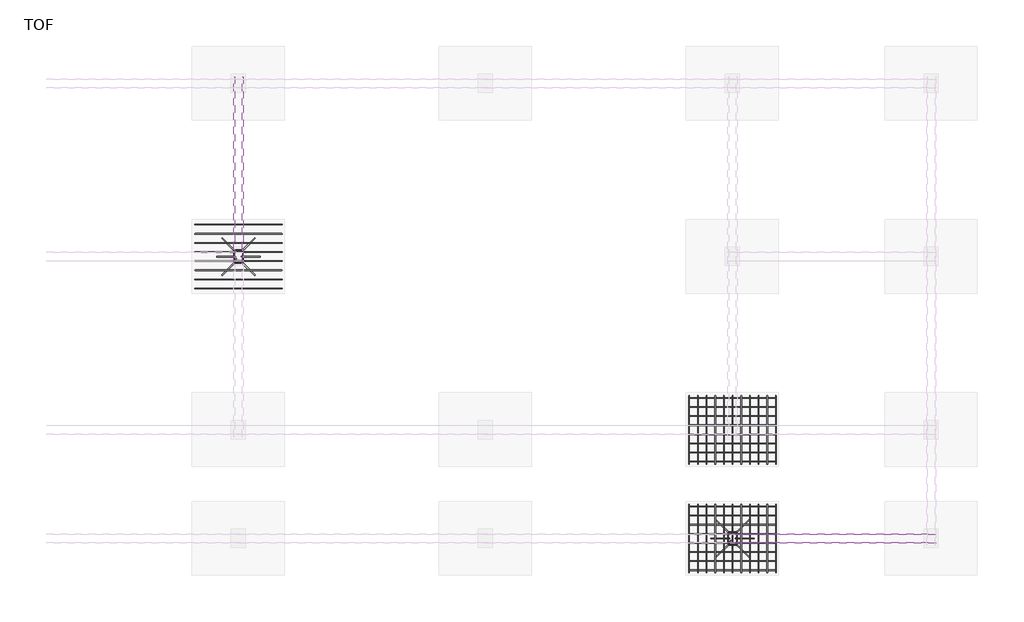
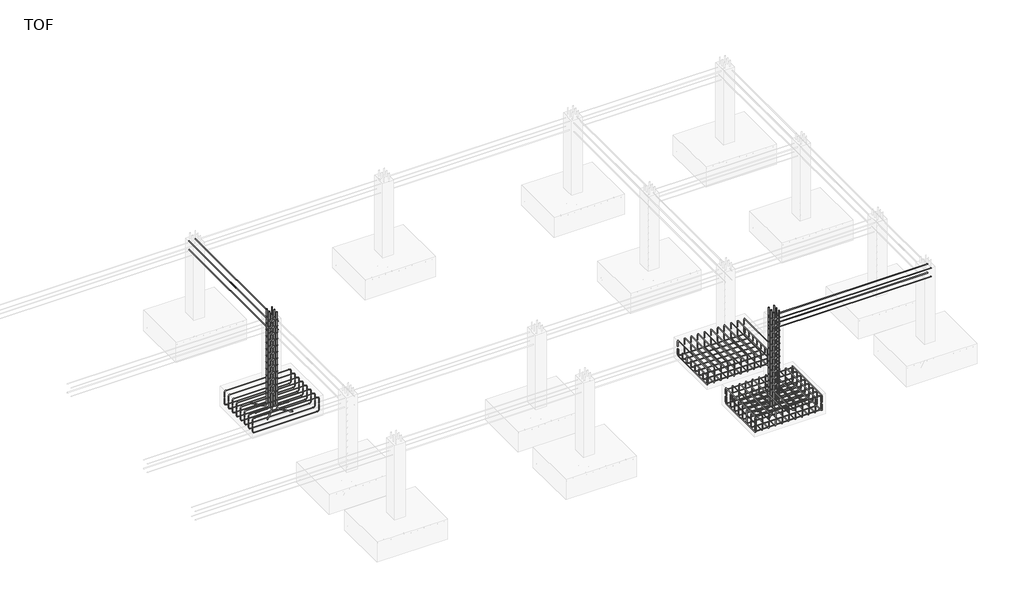
# One storey, part 6 of 10: 31 reinforcing bars.
"""IFC4 building model written with IfcOpenShell, lengths in millimetres."""

from ifc_helpers import new_model, si_unit, point, frame, origin, place, context, project, spatial, polyline, circle_curve, trimmed, segment, composite_curve, source, transform, mapped, element, save
from ifc_brep_helpers import swept_disk

model = new_model("IFC4")

# Units and contexts
model_context = context("Model", 3, world=origin())
ifc_project = project(units=[si_unit("LENGTHUNIT", "METRE", prefix="MILLI")], contexts=[model_context])

# Site, building, storey
site = spatial("IfcSite", under=ifc_project)
building = spatial("IfcBuilding", under=site)
storey = spatial("IfcBuildingStorey", under=building, Name="TOF", Elevation=-1828.8)

# Reinforcing bars
placement = place(None, origin())
reinforcing_bar_shape = source(origin(), model_context, "Body", "SolidModel", [
    swept_disk(composite_curve([segment(polyline([(10345.2782143, -14539.6267376, -2018.8), (10345.2782143, -14539.6267376, -1908.8)]), True, "CONTINUOUS"), segment(trimmed(circle_curve(frame((10345.2782143, -14574.6267376, -1908.8), z_axis=(1.0, 0.0, 0.0), x_axis=(0.0, 35.0, 0.0)), 35.0), [point((10345.2782143, -14539.6267376, -1908.8))], [point((10345.2782143, -14574.6267376, -1873.8))], True, "CARTESIAN"), True, "CONTINUOUS"), segment(polyline([(10345.2782143, -14574.6267376, -1873.8), (10345.2782143, -15614.6267376, -1873.8)]), True, "CONTINUOUS"), segment(trimmed(circle_curve(frame((10345.2782143, -15614.6267376, -1908.8), z_axis=(1.0, 0.0, 0.0), x_axis=(0.0, 0.0, 35.0)), 35.0), [point((10345.2782143, -15614.6267376, -1873.8))], [point((10345.2782143, -15649.6267376, -1908.8))], True, "CARTESIAN"), True, "CONTINUOUS"), segment(polyline([(10345.2782143, -15649.6267376, -1908.8), (10345.2782143, -15649.6267376, -2018.8)]), True, "CONTINUOUS")], self_intersect=False), 5.0),
])
element("IfcReinforcingBar", 1, at=placement, inside=storey, context=model_context, shape_type="MappedRepresentation", body=[
    mapped(reinforcing_bar_shape, transform((0.0, 0.0, 0.0), x_axis=(1.0, 0.0, 0.0), y_axis=(0.0, 1.0, 0.0), z_axis=(0.0, 0.0, 1.0))),
    mapped(reinforcing_bar_shape, transform((-141.0, 0.0, 0.0), x_axis=(1.0, 0.0, 0.0), y_axis=(0.0, 1.0, 0.0), z_axis=(0.0, 0.0, 1.0))),
    mapped(reinforcing_bar_shape, transform((-282.0, 0.0, 0.0), x_axis=(1.0, 0.0, 0.0), y_axis=(0.0, 1.0, 0.0), z_axis=(0.0, 0.0, 1.0))),
    mapped(reinforcing_bar_shape, transform((-423.0, 0.0, 0.0), x_axis=(1.0, 0.0, 0.0), y_axis=(0.0, 1.0, 0.0), z_axis=(0.0, 0.0, 1.0))),
    mapped(reinforcing_bar_shape, transform((-564.0, 0.0, 0.0), x_axis=(1.0, 0.0, 0.0), y_axis=(0.0, 1.0, 0.0), z_axis=(0.0, 0.0, 1.0))),
    mapped(reinforcing_bar_shape, transform((-705.0, 0.0, 0.0), x_axis=(1.0, 0.0, 0.0), y_axis=(0.0, 1.0, 0.0), z_axis=(0.0, 0.0, 1.0))),
    mapped(reinforcing_bar_shape, transform((-846.0, 0.0, 0.0), x_axis=(1.0, 0.0, 0.0), y_axis=(0.0, 1.0, 0.0), z_axis=(0.0, 0.0, 1.0))),
    mapped(reinforcing_bar_shape, transform((-987.0, 0.0, 0.0), x_axis=(1.0, 0.0, 0.0), y_axis=(0.0, 1.0, 0.0), z_axis=(0.0, 0.0, 1.0))),
    mapped(reinforcing_bar_shape, transform((-1128.0, 0.0, 0.0), x_axis=(1.0, 0.0, 0.0), y_axis=(0.0, 1.0, 0.0), z_axis=(0.0, 0.0, 1.0))),
    mapped(reinforcing_bar_shape, transform((-1269.0, 0.0, 0.0), x_axis=(1.0, 0.0, 0.0), y_axis=(0.0, 1.0, 0.0), z_axis=(0.0, 0.0, 1.0))),
    mapped(reinforcing_bar_shape, transform((-1410.0, 0.0, 0.0), x_axis=(1.0, 0.0, 0.0), y_axis=(0.0, 1.0, 0.0), z_axis=(0.0, 0.0, 1.0))),
])
reinforcing_bar_2_shape = source(origin(), model_context, "Body", "SolidModel", [
    swept_disk(composite_curve([segment(polyline([(10345.2782143, -15649.6267376, -2077.5233378), (10345.2782143, -15649.6267376, -2187.5233378)]), True, "CONTINUOUS"), segment(trimmed(circle_curve(frame((10345.2782143, -15614.6267376, -2187.5233378), z_axis=(1.0, 0.0, 0.0), x_axis=(0.0, -35.0, 0.0)), 35.0), [point((10345.2782143, -15649.6267376, -2187.5233378))], [point((10345.2782143, -15614.6267376, -2222.5233378))], True, "CARTESIAN"), True, "CONTINUOUS"), segment(polyline([(10345.2782143, -15614.6267376, -2222.5233378), (10345.2782143, -14574.6267376, -2222.5233378)]), True, "CONTINUOUS"), segment(trimmed(circle_curve(frame((10345.2782143, -14574.6267376, -2187.5233378), z_axis=(1.0, 0.0, 0.0), x_axis=(0.0, 0.0, -35.0)), 35.0), [point((10345.2782143, -14574.6267376, -2222.5233378))], [point((10345.2782143, -14539.6267376, -2187.5233378))], True, "CARTESIAN"), True, "CONTINUOUS"), segment(polyline([(10345.2782143, -14539.6267376, -2187.5233378), (10345.2782143, -14539.6267376, -2077.5233378)]), True, "CONTINUOUS")], self_intersect=False), 5.0),
])
element("IfcReinforcingBar", 2, at=placement, inside=storey, context=model_context, shape_type="MappedRepresentation", body=[
    mapped(reinforcing_bar_2_shape, transform((0.0, 0.0, 0.0), x_axis=(1.0, 0.0, 0.0), y_axis=(0.0, 1.0, 0.0), z_axis=(0.0, 0.0, 1.0))),
    mapped(reinforcing_bar_2_shape, transform((-141.0, 0.0, 0.0), x_axis=(1.0, 0.0, 0.0), y_axis=(0.0, 1.0, 0.0), z_axis=(0.0, 0.0, 1.0))),
    mapped(reinforcing_bar_2_shape, transform((-282.0, 0.0, 0.0), x_axis=(1.0, 0.0, 0.0), y_axis=(0.0, 1.0, 0.0), z_axis=(0.0, 0.0, 1.0))),
    mapped(reinforcing_bar_2_shape, transform((-423.0, 0.0, 0.0), x_axis=(1.0, 0.0, 0.0), y_axis=(0.0, 1.0, 0.0), z_axis=(0.0, 0.0, 1.0))),
    mapped(reinforcing_bar_2_shape, transform((-564.0, 0.0, 0.0), x_axis=(1.0, 0.0, 0.0), y_axis=(0.0, 1.0, 0.0), z_axis=(0.0, 0.0, 1.0))),
    mapped(reinforcing_bar_2_shape, transform((-705.0, 0.0, 0.0), x_axis=(1.0, 0.0, 0.0), y_axis=(0.0, 1.0, 0.0), z_axis=(0.0, 0.0, 1.0))),
    mapped(reinforcing_bar_2_shape, transform((-846.0, 0.0, 0.0), x_axis=(1.0, 0.0, 0.0), y_axis=(0.0, 1.0, 0.0), z_axis=(0.0, 0.0, 1.0))),
    mapped(reinforcing_bar_2_shape, transform((-987.0, 0.0, 0.0), x_axis=(1.0, 0.0, 0.0), y_axis=(0.0, 1.0, 0.0), z_axis=(0.0, 0.0, 1.0))),
    mapped(reinforcing_bar_2_shape, transform((-1128.0, 0.0, 0.0), x_axis=(1.0, 0.0, 0.0), y_axis=(0.0, 1.0, 0.0), z_axis=(0.0, 0.0, 1.0))),
    mapped(reinforcing_bar_2_shape, transform((-1269.0, 0.0, 0.0), x_axis=(1.0, 0.0, 0.0), y_axis=(0.0, 1.0, 0.0), z_axis=(0.0, 0.0, 1.0))),
    mapped(reinforcing_bar_2_shape, transform((-1410.0, 0.0, 0.0), x_axis=(1.0, 0.0, 0.0), y_axis=(0.0, 1.0, 0.0), z_axis=(0.0, 0.0, 1.0))),
])
reinforcing_bar_3_shape = source(origin(), model_context, "Body", "SolidModel", [
    swept_disk(composite_curve([segment(polyline([(10345.2782143, -14574.6861459, -2066.1776706), (10345.2782143, -14574.6861459, -2176.1776706)]), True, "CONTINUOUS"), segment(trimmed(circle_curve(frame((10310.2782143, -14574.6861459, -2176.1776706), z_axis=(0.0, 1.0, 0.0), x_axis=(35.0, 0.0, 0.0)), 35.0), [point((10345.2782143, -14574.6861459, -2176.1776706))], [point((10310.2782143, -14574.6861459, -2211.1776706))], True, "CARTESIAN"), True, "CONTINUOUS"), segment(polyline([(10310.2782143, -14574.6861459, -2211.1776706), (8970.2782143, -14574.6861459, -2211.1776706)]), True, "CONTINUOUS"), segment(trimmed(circle_curve(frame((8970.2782143, -14574.6861459, -2176.1776706), z_axis=(0.0, 1.0, 0.0), x_axis=(0.0, 0.0, -35.0)), 35.0), [point((8970.2782143, -14574.6861459, -2211.1776706))], [point((8935.2782143, -14574.6861459, -2176.1776706))], True, "CARTESIAN"), True, "CONTINUOUS"), segment(polyline([(8935.2782143, -14574.6861459, -2176.1776706), (8935.2782143, -14574.6861459, -2066.1776706)]), True, "CONTINUOUS")], self_intersect=False), 5.0),
])
element("IfcReinforcingBar", 3, at=placement, inside=storey, context=model_context, shape_type="MappedRepresentation", body=[
    mapped(reinforcing_bar_3_shape, transform((0.0, 0.0, 0.0), x_axis=(1.0, 0.0, 0.0), y_axis=(0.0, 1.0, 0.0), z_axis=(0.0, 0.0, 1.0))),
    mapped(reinforcing_bar_3_shape, transform((0.0, -148.0321606, 0.0), x_axis=(1.0, 0.0, 0.0), y_axis=(0.0, 1.0, 0.0), z_axis=(0.0, 0.0, 1.0))),
    mapped(reinforcing_bar_3_shape, transform((0.0, -296.0643211, 0.0), x_axis=(1.0, 0.0, 0.0), y_axis=(0.0, 1.0, 0.0), z_axis=(0.0, 0.0, 1.0))),
    mapped(reinforcing_bar_3_shape, transform((0.0, -444.0964817, 0.0), x_axis=(1.0, 0.0, 0.0), y_axis=(0.0, 1.0, 0.0), z_axis=(0.0, 0.0, 1.0))),
    mapped(reinforcing_bar_3_shape, transform((0.0, -592.1286423, 0.0), x_axis=(1.0, 0.0, 0.0), y_axis=(0.0, 1.0, 0.0), z_axis=(0.0, 0.0, 1.0))),
    mapped(reinforcing_bar_3_shape, transform((0.0, -740.1608029, 0.0), x_axis=(1.0, 0.0, 0.0), y_axis=(0.0, 1.0, 0.0), z_axis=(0.0, 0.0, 1.0))),
    mapped(reinforcing_bar_3_shape, transform((0.0, -888.1929634, 0.0), x_axis=(1.0, 0.0, 0.0), y_axis=(0.0, 1.0, 0.0), z_axis=(0.0, 0.0, 1.0))),
    mapped(reinforcing_bar_3_shape, transform((0.0, -1036.225124, 0.0), x_axis=(1.0, 0.0, 0.0), y_axis=(0.0, 1.0, 0.0), z_axis=(0.0, 0.0, 1.0))),
])
reinforcing_bar_4_shape = source(origin(), model_context, "Body", "SolidModel", [
    swept_disk(composite_curve([segment(polyline([(10345.2782143, -15610.9112699, -2039.256778), (10345.2782143, -15610.9112699, -1929.256778)]), True, "CONTINUOUS"), segment(trimmed(circle_curve(frame((10310.2782143, -15610.9112699, -1929.256778), z_axis=(0.0, -1.0, 0.0), x_axis=(35.0, 0.0, 0.0)), 35.0), [point((10345.2782143, -15610.9112699, -1929.256778))], [point((10310.2782143, -15610.9112699, -1894.256778))], True, "CARTESIAN"), True, "CONTINUOUS"), segment(polyline([(10310.2782143, -15610.9112699, -1894.256778), (8970.2782143, -15610.9112699, -1894.256778)]), True, "CONTINUOUS"), segment(trimmed(circle_curve(frame((8970.2782143, -15610.9112699, -1929.256778), z_axis=(0.0, -1.0, 0.0), x_axis=(0.0, 0.0, 35.0)), 35.0), [point((8970.2782143, -15610.9112699, -1894.256778))], [point((8935.2782143, -15610.9112699, -1929.256778))], True, "CARTESIAN"), True, "CONTINUOUS"), segment(polyline([(8935.2782143, -15610.9112699, -1929.256778), (8935.2782143, -15610.9112699, -2039.256778)]), True, "CONTINUOUS")], self_intersect=False), 5.0),
])
element("IfcReinforcingBar", 4, at=placement, inside=storey, context=model_context, shape_type="MappedRepresentation", body=[
    mapped(reinforcing_bar_4_shape, transform((0.0, 0.0, 0.0), x_axis=(1.0, 0.0, 0.0), y_axis=(0.0, 1.0, 0.0), z_axis=(0.0, 0.0, 1.0))),
    mapped(reinforcing_bar_4_shape, transform((0.0, 148.0321606, 0.0), x_axis=(1.0, 0.0, 0.0), y_axis=(0.0, 1.0, 0.0), z_axis=(0.0, 0.0, 1.0))),
    mapped(reinforcing_bar_4_shape, transform((0.0, 296.0643211, 0.0), x_axis=(1.0, 0.0, 0.0), y_axis=(0.0, 1.0, 0.0), z_axis=(0.0, 0.0, 1.0))),
    mapped(reinforcing_bar_4_shape, transform((0.0, 444.0964817, 0.0), x_axis=(1.0, 0.0, 0.0), y_axis=(0.0, 1.0, 0.0), z_axis=(0.0, 0.0, 1.0))),
    mapped(reinforcing_bar_4_shape, transform((0.0, 592.1286423, 0.0), x_axis=(1.0, 0.0, 0.0), y_axis=(0.0, 1.0, 0.0), z_axis=(0.0, 0.0, 1.0))),
    mapped(reinforcing_bar_4_shape, transform((0.0, 740.1608029, 0.0), x_axis=(1.0, 0.0, 0.0), y_axis=(0.0, 1.0, 0.0), z_axis=(0.0, 0.0, 1.0))),
    mapped(reinforcing_bar_4_shape, transform((0.0, 888.1929634, 0.0), x_axis=(1.0, 0.0, 0.0), y_axis=(0.0, 1.0, 0.0), z_axis=(0.0, 0.0, 1.0))),
    mapped(reinforcing_bar_4_shape, transform((0.0, 1036.225124, 0.0), x_axis=(1.0, 0.0, 0.0), y_axis=(0.0, 1.0, 0.0), z_axis=(0.0, 0.0, 1.0))),
])
reinforcing_bar_5_shape = source(origin(), model_context, "Body", "SolidModel", [
    swept_disk(composite_curve([segment(polyline([(10345.2782143, -12774.6267376, -2018.8), (10345.2782143, -12774.6267376, -1908.8)]), True, "CONTINUOUS"), segment(trimmed(circle_curve(frame((10345.2782143, -12809.6267376, -1908.8), z_axis=(1.0, 0.0, 0.0), x_axis=(0.0, 35.0, 0.0)), 35.0), [point((10345.2782143, -12774.6267376, -1908.8))], [point((10345.2782143, -12809.6267376, -1873.8))], True, "CARTESIAN"), True, "CONTINUOUS"), segment(polyline([(10345.2782143, -12809.6267376, -1873.8), (10345.2782143, -13849.6267376, -1873.8)]), True, "CONTINUOUS"), segment(trimmed(circle_curve(frame((10345.2782143, -13849.6267376, -1908.8), z_axis=(1.0, 0.0, 0.0), x_axis=(0.0, 0.0, 35.0)), 35.0), [point((10345.2782143, -13849.6267376, -1873.8))], [point((10345.2782143, -13884.6267376, -1908.8))], True, "CARTESIAN"), True, "CONTINUOUS"), segment(polyline([(10345.2782143, -13884.6267376, -1908.8), (10345.2782143, -13884.6267376, -2018.8)]), True, "CONTINUOUS")], self_intersect=False), 5.0),
])
element("IfcReinforcingBar", 5, at=placement, inside=storey, context=model_context, shape_type="MappedRepresentation", body=[
    mapped(reinforcing_bar_5_shape, transform((0.0, 0.0, 0.0), x_axis=(1.0, 0.0, 0.0), y_axis=(0.0, 1.0, 0.0), z_axis=(0.0, 0.0, 1.0))),
    mapped(reinforcing_bar_5_shape, transform((-141.0, 0.0, 0.0), x_axis=(1.0, 0.0, 0.0), y_axis=(0.0, 1.0, 0.0), z_axis=(0.0, 0.0, 1.0))),
    mapped(reinforcing_bar_5_shape, transform((-282.0, 0.0, 0.0), x_axis=(1.0, 0.0, 0.0), y_axis=(0.0, 1.0, 0.0), z_axis=(0.0, 0.0, 1.0))),
    mapped(reinforcing_bar_5_shape, transform((-423.0, 0.0, 0.0), x_axis=(1.0, 0.0, 0.0), y_axis=(0.0, 1.0, 0.0), z_axis=(0.0, 0.0, 1.0))),
    mapped(reinforcing_bar_5_shape, transform((-564.0, 0.0, 0.0), x_axis=(1.0, 0.0, 0.0), y_axis=(0.0, 1.0, 0.0), z_axis=(0.0, 0.0, 1.0))),
    mapped(reinforcing_bar_5_shape, transform((-705.0, 0.0, 0.0), x_axis=(1.0, 0.0, 0.0), y_axis=(0.0, 1.0, 0.0), z_axis=(0.0, 0.0, 1.0))),
    mapped(reinforcing_bar_5_shape, transform((-846.0, 0.0, 0.0), x_axis=(1.0, 0.0, 0.0), y_axis=(0.0, 1.0, 0.0), z_axis=(0.0, 0.0, 1.0))),
    mapped(reinforcing_bar_5_shape, transform((-987.0, 0.0, 0.0), x_axis=(1.0, 0.0, 0.0), y_axis=(0.0, 1.0, 0.0), z_axis=(0.0, 0.0, 1.0))),
    mapped(reinforcing_bar_5_shape, transform((-1128.0, 0.0, 0.0), x_axis=(1.0, 0.0, 0.0), y_axis=(0.0, 1.0, 0.0), z_axis=(0.0, 0.0, 1.0))),
    mapped(reinforcing_bar_5_shape, transform((-1269.0, 0.0, 0.0), x_axis=(1.0, 0.0, 0.0), y_axis=(0.0, 1.0, 0.0), z_axis=(0.0, 0.0, 1.0))),
    mapped(reinforcing_bar_5_shape, transform((-1410.0, 0.0, 0.0), x_axis=(1.0, 0.0, 0.0), y_axis=(0.0, 1.0, 0.0), z_axis=(0.0, 0.0, 1.0))),
])
reinforcing_bar_6_shape = source(origin(), model_context, "Body", "SolidModel", [
    swept_disk(composite_curve([segment(polyline([(10345.2782143, -13884.6267376, -2077.5233378), (10345.2782143, -13884.6267376, -2187.5233378)]), True, "CONTINUOUS"), segment(trimmed(circle_curve(frame((10345.2782143, -13849.6267376, -2187.5233378), z_axis=(1.0, 0.0, 0.0), x_axis=(0.0, -35.0, 0.0)), 35.0), [point((10345.2782143, -13884.6267376, -2187.5233378))], [point((10345.2782143, -13849.6267376, -2222.5233378))], True, "CARTESIAN"), True, "CONTINUOUS"), segment(polyline([(10345.2782143, -13849.6267376, -2222.5233378), (10345.2782143, -12809.6267376, -2222.5233378)]), True, "CONTINUOUS"), segment(trimmed(circle_curve(frame((10345.2782143, -12809.6267376, -2187.5233378), z_axis=(1.0, 0.0, 0.0), x_axis=(0.0, 0.0, -35.0)), 35.0), [point((10345.2782143, -12809.6267376, -2222.5233378))], [point((10345.2782143, -12774.6267376, -2187.5233378))], True, "CARTESIAN"), True, "CONTINUOUS"), segment(polyline([(10345.2782143, -12774.6267376, -2187.5233378), (10345.2782143, -12774.6267376, -2077.5233378)]), True, "CONTINUOUS")], self_intersect=False), 5.0),
])
element("IfcReinforcingBar", 6, at=placement, inside=storey, context=model_context, shape_type="MappedRepresentation", body=[
    mapped(reinforcing_bar_6_shape, transform((0.0, 0.0, 0.0), x_axis=(1.0, 0.0, 0.0), y_axis=(0.0, 1.0, 0.0), z_axis=(0.0, 0.0, 1.0))),
    mapped(reinforcing_bar_6_shape, transform((-141.0, 0.0, 0.0), x_axis=(1.0, 0.0, 0.0), y_axis=(0.0, 1.0, 0.0), z_axis=(0.0, 0.0, 1.0))),
    mapped(reinforcing_bar_6_shape, transform((-282.0, 0.0, 0.0), x_axis=(1.0, 0.0, 0.0), y_axis=(0.0, 1.0, 0.0), z_axis=(0.0, 0.0, 1.0))),
    mapped(reinforcing_bar_6_shape, transform((-423.0, 0.0, 0.0), x_axis=(1.0, 0.0, 0.0), y_axis=(0.0, 1.0, 0.0), z_axis=(0.0, 0.0, 1.0))),
    mapped(reinforcing_bar_6_shape, transform((-564.0, 0.0, 0.0), x_axis=(1.0, 0.0, 0.0), y_axis=(0.0, 1.0, 0.0), z_axis=(0.0, 0.0, 1.0))),
    mapped(reinforcing_bar_6_shape, transform((-705.0, 0.0, 0.0), x_axis=(1.0, 0.0, 0.0), y_axis=(0.0, 1.0, 0.0), z_axis=(0.0, 0.0, 1.0))),
    mapped(reinforcing_bar_6_shape, transform((-846.0, 0.0, 0.0), x_axis=(1.0, 0.0, 0.0), y_axis=(0.0, 1.0, 0.0), z_axis=(0.0, 0.0, 1.0))),
    mapped(reinforcing_bar_6_shape, transform((-987.0, 0.0, 0.0), x_axis=(1.0, 0.0, 0.0), y_axis=(0.0, 1.0, 0.0), z_axis=(0.0, 0.0, 1.0))),
    mapped(reinforcing_bar_6_shape, transform((-1128.0, 0.0, 0.0), x_axis=(1.0, 0.0, 0.0), y_axis=(0.0, 1.0, 0.0), z_axis=(0.0, 0.0, 1.0))),
    mapped(reinforcing_bar_6_shape, transform((-1269.0, 0.0, 0.0), x_axis=(1.0, 0.0, 0.0), y_axis=(0.0, 1.0, 0.0), z_axis=(0.0, 0.0, 1.0))),
    mapped(reinforcing_bar_6_shape, transform((-1410.0, 0.0, 0.0), x_axis=(1.0, 0.0, 0.0), y_axis=(0.0, 1.0, 0.0), z_axis=(0.0, 0.0, 1.0))),
])
reinforcing_bar_7_shape = source(origin(), model_context, "Body", "SolidModel", [
    swept_disk(composite_curve([segment(polyline([(10345.2782143, -12809.6861459, -2066.1776706), (10345.2782143, -12809.6861459, -2176.1776706)]), True, "CONTINUOUS"), segment(trimmed(circle_curve(frame((10310.2782143, -12809.6861459, -2176.1776706), z_axis=(0.0, 1.0, 0.0), x_axis=(35.0, 0.0, 0.0)), 35.0), [point((10345.2782143, -12809.6861459, -2176.1776706))], [point((10310.2782143, -12809.6861459, -2211.1776706))], True, "CARTESIAN"), True, "CONTINUOUS"), segment(polyline([(10310.2782143, -12809.6861459, -2211.1776706), (8970.2782143, -12809.6861459, -2211.1776706)]), True, "CONTINUOUS"), segment(trimmed(circle_curve(frame((8970.2782143, -12809.6861459, -2176.1776706), z_axis=(0.0, 1.0, 0.0), x_axis=(0.0, 0.0, -35.0)), 35.0), [point((8970.2782143, -12809.6861459, -2211.1776706))], [point((8935.2782143, -12809.6861459, -2176.1776706))], True, "CARTESIAN"), True, "CONTINUOUS"), segment(polyline([(8935.2782143, -12809.6861459, -2176.1776706), (8935.2782143, -12809.6861459, -2066.1776706)]), True, "CONTINUOUS")], self_intersect=False), 5.0),
])
element("IfcReinforcingBar", 7, at=placement, inside=storey, context=model_context, shape_type="MappedRepresentation", body=[
    mapped(reinforcing_bar_7_shape, transform((0.0, 0.0, 0.0), x_axis=(1.0, 0.0, 0.0), y_axis=(0.0, 1.0, 0.0), z_axis=(0.0, 0.0, 1.0))),
    mapped(reinforcing_bar_7_shape, transform((0.0, -148.0321606, 0.0), x_axis=(1.0, 0.0, 0.0), y_axis=(0.0, 1.0, 0.0), z_axis=(0.0, 0.0, 1.0))),
    mapped(reinforcing_bar_7_shape, transform((0.0, -296.0643211, 0.0), x_axis=(1.0, 0.0, 0.0), y_axis=(0.0, 1.0, 0.0), z_axis=(0.0, 0.0, 1.0))),
    mapped(reinforcing_bar_7_shape, transform((0.0, -444.0964817, 0.0), x_axis=(1.0, 0.0, 0.0), y_axis=(0.0, 1.0, 0.0), z_axis=(0.0, 0.0, 1.0))),
    mapped(reinforcing_bar_7_shape, transform((0.0, -592.1286423, 0.0), x_axis=(1.0, 0.0, 0.0), y_axis=(0.0, 1.0, 0.0), z_axis=(0.0, 0.0, 1.0))),
    mapped(reinforcing_bar_7_shape, transform((0.0, -740.1608029, 0.0), x_axis=(1.0, 0.0, 0.0), y_axis=(0.0, 1.0, 0.0), z_axis=(0.0, 0.0, 1.0))),
    mapped(reinforcing_bar_7_shape, transform((0.0, -888.1929634, 0.0), x_axis=(1.0, 0.0, 0.0), y_axis=(0.0, 1.0, 0.0), z_axis=(0.0, 0.0, 1.0))),
    mapped(reinforcing_bar_7_shape, transform((0.0, -1036.225124, 0.0), x_axis=(1.0, 0.0, 0.0), y_axis=(0.0, 1.0, 0.0), z_axis=(0.0, 0.0, 1.0))),
])
reinforcing_bar_8_shape = source(origin(), model_context, "Body", "SolidModel", [
    swept_disk(composite_curve([segment(polyline([(2315.2782143, -9994.6861459, -2066.1776706), (2315.2782143, -9994.6861459, -2176.1776706)]), True, "CONTINUOUS"), segment(trimmed(circle_curve(frame((2280.2782143, -9994.6861459, -2176.1776706), z_axis=(0.0, 1.0, 0.0), x_axis=(35.0, 0.0, 0.0)), 35.0), [point((2315.2782143, -9994.6861459, -2176.1776706))], [point((2280.2782143, -9994.6861459, -2211.1776706))], True, "CARTESIAN"), True, "CONTINUOUS"), segment(polyline([(2280.2782143, -9994.6861459, -2211.1776706), (940.2782143, -9994.6861459, -2211.1776706)]), True, "CONTINUOUS"), segment(trimmed(circle_curve(frame((940.2782143, -9994.6861459, -2176.1776706), z_axis=(0.0, 1.0, 0.0), x_axis=(0.0, 0.0, -35.0)), 35.0), [point((940.2782143, -9994.6861459, -2211.1776706))], [point((905.2782143, -9994.6861459, -2176.1776706))], True, "CARTESIAN"), True, "CONTINUOUS"), segment(polyline([(905.2782143, -9994.6861459, -2176.1776706), (905.2782143, -9994.6861459, -2066.1776706)]), True, "CONTINUOUS")], self_intersect=False), 5.0),
])
element("IfcReinforcingBar", 8, at=placement, inside=storey, context=model_context, shape_type="MappedRepresentation", body=[
    mapped(reinforcing_bar_8_shape, transform((0.0, 0.0, 0.0), x_axis=(1.0, 0.0, 0.0), y_axis=(0.0, 1.0, 0.0), z_axis=(0.0, 0.0, 1.0))),
    mapped(reinforcing_bar_8_shape, transform((0.0, -148.0321606, 0.0), x_axis=(1.0, 0.0, 0.0), y_axis=(0.0, 1.0, 0.0), z_axis=(0.0, 0.0, 1.0))),
    mapped(reinforcing_bar_8_shape, transform((0.0, -296.0643211, 0.0), x_axis=(1.0, 0.0, 0.0), y_axis=(0.0, 1.0, 0.0), z_axis=(0.0, 0.0, 1.0))),
    mapped(reinforcing_bar_8_shape, transform((0.0, -444.0964817, 0.0), x_axis=(1.0, 0.0, 0.0), y_axis=(0.0, 1.0, 0.0), z_axis=(0.0, 0.0, 1.0))),
    mapped(reinforcing_bar_8_shape, transform((0.0, -592.1286423, 0.0), x_axis=(1.0, 0.0, 0.0), y_axis=(0.0, 1.0, 0.0), z_axis=(0.0, 0.0, 1.0))),
    mapped(reinforcing_bar_8_shape, transform((0.0, -740.1608029, 0.0), x_axis=(1.0, 0.0, 0.0), y_axis=(0.0, 1.0, 0.0), z_axis=(0.0, 0.0, 1.0))),
    mapped(reinforcing_bar_8_shape, transform((0.0, -888.1929634, 0.0), x_axis=(1.0, 0.0, 0.0), y_axis=(0.0, 1.0, 0.0), z_axis=(0.0, 0.0, 1.0))),
    mapped(reinforcing_bar_8_shape, transform((0.0, -1036.225124, 0.0), x_axis=(1.0, 0.0, 0.0), y_axis=(0.0, 1.0, 0.0), z_axis=(0.0, 0.0, 1.0))),
])
reinforcing_bar_9_shape = source(origin(), model_context, "Body", "SolidModel", [
    swept_disk(composite_curve([segment(polyline([(2315.2782143, -11030.9112699, -2039.256778), (2315.2782143, -11030.9112699, -1929.256778)]), True, "CONTINUOUS"), segment(trimmed(circle_curve(frame((2280.2782143, -11030.9112699, -1929.256778), z_axis=(0.0, -1.0, 0.0), x_axis=(35.0, 0.0, 0.0)), 35.0), [point((2315.2782143, -11030.9112699, -1929.256778))], [point((2280.2782143, -11030.9112699, -1894.256778))], True, "CARTESIAN"), True, "CONTINUOUS"), segment(polyline([(2280.2782143, -11030.9112699, -1894.256778), (940.2782143, -11030.9112699, -1894.256778)]), True, "CONTINUOUS"), segment(trimmed(circle_curve(frame((940.2782143, -11030.9112699, -1929.256778), z_axis=(0.0, -1.0, 0.0), x_axis=(0.0, 0.0, 35.0)), 35.0), [point((940.2782143, -11030.9112699, -1894.256778))], [point((905.2782143, -11030.9112699, -1929.256778))], True, "CARTESIAN"), True, "CONTINUOUS"), segment(polyline([(905.2782143, -11030.9112699, -1929.256778), (905.2782143, -11030.9112699, -2039.256778)]), True, "CONTINUOUS")], self_intersect=False), 5.0),
])
element("IfcReinforcingBar", 9, at=placement, inside=storey, context=model_context, shape_type="MappedRepresentation", body=[
    mapped(reinforcing_bar_9_shape, transform((0.0, 0.0, 0.0), x_axis=(1.0, 0.0, 0.0), y_axis=(0.0, 1.0, 0.0), z_axis=(0.0, 0.0, 1.0))),
    mapped(reinforcing_bar_9_shape, transform((0.0, 148.0321606, 0.0), x_axis=(1.0, 0.0, 0.0), y_axis=(0.0, 1.0, 0.0), z_axis=(0.0, 0.0, 1.0))),
    mapped(reinforcing_bar_9_shape, transform((0.0, 296.0643211, 0.0), x_axis=(1.0, 0.0, 0.0), y_axis=(0.0, 1.0, 0.0), z_axis=(0.0, 0.0, 1.0))),
    mapped(reinforcing_bar_9_shape, transform((0.0, 444.0964817, 0.0), x_axis=(1.0, 0.0, 0.0), y_axis=(0.0, 1.0, 0.0), z_axis=(0.0, 0.0, 1.0))),
    mapped(reinforcing_bar_9_shape, transform((0.0, 592.1286423, 0.0), x_axis=(1.0, 0.0, 0.0), y_axis=(0.0, 1.0, 0.0), z_axis=(0.0, 0.0, 1.0))),
    mapped(reinforcing_bar_9_shape, transform((0.0, 740.1608029, 0.0), x_axis=(1.0, 0.0, 0.0), y_axis=(0.0, 1.0, 0.0), z_axis=(0.0, 0.0, 1.0))),
    mapped(reinforcing_bar_9_shape, transform((0.0, 888.1929634, 0.0), x_axis=(1.0, 0.0, 0.0), y_axis=(0.0, 1.0, 0.0), z_axis=(0.0, 0.0, 1.0))),
    mapped(reinforcing_bar_9_shape, transform((0.0, 1036.225124, 0.0), x_axis=(1.0, 0.0, 0.0), y_axis=(0.0, 1.0, 0.0), z_axis=(0.0, 0.0, 1.0))),
])
reinforcing_bar_10_shape = source(origin(), model_context, "Body", "SolidModel", [
    swept_disk(composite_curve([segment(polyline([(9610.248777, -15125.7150493, -1784.8), (9576.3076515, -15159.6561748, -1784.8)]), True, "CONTINUOUS"), segment(trimmed(circle_curve(frame((9593.2782143, -15176.6267376, -1784.8), z_axis=(0.0, 0.0, 1.0), x_axis=(-16.970562800001062, 16.970562799999243, 0.0)), 24.0), [point((9576.3076515, -15159.6561748, -1784.8))], [point((9593.2782143, -15200.6267376, -1784.8))], True, "CARTESIAN"), True, "CONTINUOUS"), segment(polyline([(9593.2782143, -15200.6267376, -1784.8), (9687.2782143, -15200.6267376, -1784.8)]), True, "CONTINUOUS"), segment(trimmed(circle_curve(frame((9687.2782143, -15176.6267376, -1784.8), z_axis=(0.0, 0.0, 1.0), x_axis=(0.0, -24.0, 0.0)), 24.0), [point((9687.2782143, -15200.6267376, -1784.8))], [point((9711.2782143, -15176.6267376, -1784.8))], True, "CARTESIAN"), True, "CONTINUOUS"), segment(polyline([(9711.2782143, -15176.6267376, -1784.8), (9711.2782143, -15012.6267376, -1784.8)]), True, "CONTINUOUS"), segment(trimmed(circle_curve(frame((9687.3162115, -15012.6267376, -1786.149972), z_axis=(-0.05624883273897078, 0.0, 0.9984167811167355), x_axis=(23.962002800000846, 0.0, 1.3499719999999797)), 24.0), [point((9711.2782143, -15012.6267376, -1784.8))], [point((9687.3162115, -14988.6267376, -1786.149972))], True, "CARTESIAN"), True, "CONTINUOUS"), segment(polyline([(9687.3162115, -14988.6267376, -1786.149972), (9593.240217, -14988.6267376, -1791.450028)]), True, "CONTINUOUS"), segment(trimmed(circle_curve(frame((9593.240217, -15012.6267376, -1791.450028), z_axis=(-0.05624883273897078, 0.0, 0.9984167811167355), x_axis=(0.0, 24.0, 0.0)), 24.0), [point((9593.240217, -14988.6267376, -1791.450028))], [point((9569.2782143, -15012.6267376, -1792.8))], True, "CARTESIAN"), True, "CONTINUOUS"), segment(polyline([(9569.2782143, -15012.6267376, -1792.8), (9569.2782143, -15176.6267376, -1792.8)]), True, "CONTINUOUS"), segment(trimmed(circle_curve(frame((9593.2782143, -15176.6267376, -1792.8), z_axis=(0.0, 0.0, 1.0), x_axis=(-24.0, 0.0, 0.0)), 24.0), [point((9569.2782143, -15176.6267376, -1792.8))], [point((9610.248777, -15193.5973003, -1792.8))], True, "CARTESIAN"), True, "CONTINUOUS"), segment(polyline([(9610.248777, -15193.5973003, -1792.8), (9644.1899025, -15159.6561748, -1792.8)]), True, "CONTINUOUS")], self_intersect=False), 4.0),
])
element("IfcReinforcingBar", 10, at=placement, inside=storey, context=model_context, shape_type="MappedRepresentation", body=[
    mapped(reinforcing_bar_10_shape, transform((0.0, 0.0, 0.0), x_axis=(1.0, 0.0, 0.0), y_axis=(0.0, 1.0, 0.0), z_axis=(0.0, 0.0, 1.0))),
    mapped(reinforcing_bar_10_shape, transform((0.0, 0.0, 145.9395608), x_axis=(1.0, 0.0, 0.0), y_axis=(0.0, 1.0, 0.0), z_axis=(0.0, 0.0, 1.0))),
    mapped(reinforcing_bar_10_shape, transform((0.0, 0.0, 291.8791216), x_axis=(1.0, 0.0, 0.0), y_axis=(0.0, 1.0, 0.0), z_axis=(0.0, 0.0, 1.0))),
    mapped(reinforcing_bar_10_shape, transform((0.0, 0.0, 437.8186825), x_axis=(1.0, 0.0, 0.0), y_axis=(0.0, 1.0, 0.0), z_axis=(0.0, 0.0, 1.0))),
    mapped(reinforcing_bar_10_shape, transform((0.0, 0.0, 583.7582433), x_axis=(1.0, 0.0, 0.0), y_axis=(0.0, 1.0, 0.0), z_axis=(0.0, 0.0, 1.0))),
    mapped(reinforcing_bar_10_shape, transform((0.0, 0.0, 729.6978041), x_axis=(1.0, 0.0, 0.0), y_axis=(0.0, 1.0, 0.0), z_axis=(0.0, 0.0, 1.0))),
    mapped(reinforcing_bar_10_shape, transform((0.0, 0.0, 875.6373649), x_axis=(1.0, 0.0, 0.0), y_axis=(0.0, 1.0, 0.0), z_axis=(0.0, 0.0, 1.0))),
    mapped(reinforcing_bar_10_shape, transform((0.0, 0.0, 1021.5769258), x_axis=(1.0, 0.0, 0.0), y_axis=(0.0, 1.0, 0.0), z_axis=(0.0, 0.0, 1.0))),
    mapped(reinforcing_bar_10_shape, transform((0.0, 0.0, 1167.5164866), x_axis=(1.0, 0.0, 0.0), y_axis=(0.0, 1.0, 0.0), z_axis=(0.0, 0.0, 1.0))),
    mapped(reinforcing_bar_10_shape, transform((0.0, 0.0, 1313.4560474), x_axis=(1.0, 0.0, 0.0), y_axis=(0.0, 1.0, 0.0), z_axis=(0.0, 0.0, 1.0))),
    mapped(reinforcing_bar_10_shape, transform((0.0, 0.0, 1459.3956082), x_axis=(1.0, 0.0, 0.0), y_axis=(0.0, 1.0, 0.0), z_axis=(0.0, 0.0, 1.0))),
    mapped(reinforcing_bar_10_shape, transform((0.0, 0.0, 1605.3351691), x_axis=(1.0, 0.0, 0.0), y_axis=(0.0, 1.0, 0.0), z_axis=(0.0, 0.0, 1.0))),
])
element("IfcReinforcingBar", 11, at=placement, inside=storey, context=model_context, shape_type="SolidModel", body=[
    swept_disk(composite_curve([segment(polyline([(9695.884816, -15185.2333393, -20.0), (9695.884816, -15185.2333393, -2138.7824747)]), True, "CONTINUOUS"), segment(trimmed(circle_curve(frame((9735.1292424, -15224.4777657, -2138.7824747), z_axis=(-0.7071067811865545, -0.7071067811865406, 0.0), x_axis=(-39.24442640000052, 39.2444263999987, 0.0)), 55.5), [point((9695.884816, -15185.2333393, -2138.7824747))], [point((9735.1292424, -15224.4777657, -2194.2824747))], True, "CARTESIAN"), True, "CONTINUOUS"), segment(polyline([(9735.1292424, -15224.4777657, -2194.2824747), (9907.5083915, -15396.8569148, -2194.2824747)]), True, "CONTINUOUS")], self_intersect=False), 8.0),
])
element("IfcReinforcingBar", 12, at=placement, inside=storey, context=model_context, shape_type="SolidModel", body=[
    swept_disk(composite_curve([segment(polyline([(9695.934816, -15094.6267376, -20.0), (9695.934816, -15094.6267376, -2138.7824747)]), True, "CONTINUOUS"), segment(trimmed(circle_curve(frame((9751.434816, -15094.6267376, -2138.7824747), z_axis=(0.0, -1.0, 0.0), x_axis=(-55.5, 0.0, 0.0)), 55.5), [point((9695.934816, -15094.6267376, -2138.7824747))], [point((9751.434816, -15094.6267376, -2194.2824747))], True, "CARTESIAN"), True, "CONTINUOUS"), segment(polyline([(9751.434816, -15094.6267376, -2194.2824747), (9995.1657466, -15094.6267376, -2194.2824747)]), True, "CONTINUOUS")], self_intersect=False), 8.0),
])
element("IfcReinforcingBar", 13, at=placement, inside=storey, context=model_context, shape_type="SolidModel", body=[
    swept_disk(composite_curve([segment(polyline([(9695.884816, -15004.0201359, -20.0), (9695.884816, -15004.0201359, -2138.7824747)]), True, "CONTINUOUS"), segment(trimmed(circle_curve(frame((9735.1292424, -14964.7757095, -2138.7824747), z_axis=(0.7071067811865545, -0.7071067811865407, 0.0), x_axis=(-39.24442640000052, -39.24442640000052, 0.0)), 55.5), [point((9695.884816, -15004.0201359, -2138.7824747))], [point((9735.1292424, -14964.7757095, -2194.2824747))], True, "CARTESIAN"), True, "CONTINUOUS"), segment(polyline([(9735.1292424, -14964.7757095, -2194.2824747), (9907.5083915, -14792.3965603, -2194.2824747)]), True, "CONTINUOUS")], self_intersect=False), 8.0),
])
element("IfcReinforcingBar", 14, at=placement, inside=storey, context=model_context, shape_type="SolidModel", body=[
    swept_disk(composite_curve([segment(polyline([(9584.6716126, -15185.2333393, -20.0), (9584.6716126, -15185.2333393, -2138.7824747)]), True, "CONTINUOUS"), segment(trimmed(circle_curve(frame((9545.4271862, -15224.4777657, -2138.7824747), z_axis=(-0.7071067811865517, 0.7071067811865434, 0.0), x_axis=(39.2444263999987, 39.2444263999987, 0.0)), 55.5), [point((9584.6716126, -15185.2333393, -2138.7824747))], [point((9545.4271862, -15224.4777657, -2194.2824747))], True, "CARTESIAN"), True, "CONTINUOUS"), segment(polyline([(9545.4271862, -15224.4777657, -2194.2824747), (9373.048037, -15396.8569148, -2194.2824747)]), True, "CONTINUOUS")], self_intersect=False), 8.0),
])
element("IfcReinforcingBar", 15, at=placement, inside=storey, context=model_context, shape_type="SolidModel", body=[
    swept_disk(composite_curve([segment(polyline([(9584.6216126, -15094.6267376, -20.0), (9584.6216126, -15094.6267376, -2138.7824747)]), True, "CONTINUOUS"), segment(trimmed(circle_curve(frame((9529.1216126, -15094.6267376, -2138.7824747), z_axis=(0.0, 1.0, 0.0), x_axis=(55.5, 0.0, 0.0)), 55.5), [point((9584.6216126, -15094.6267376, -2138.7824747))], [point((9529.1216126, -15094.6267376, -2194.2824747))], True, "CARTESIAN"), True, "CONTINUOUS"), segment(polyline([(9529.1216126, -15094.6267376, -2194.2824747), (9285.3906819, -15094.6267376, -2194.2824747)]), True, "CONTINUOUS")], self_intersect=False), 8.0),
])
element("IfcReinforcingBar", 16, at=placement, inside=storey, context=model_context, shape_type="SolidModel", body=[
    swept_disk(composite_curve([segment(polyline([(9584.6716126, -15004.0201359, -20.0), (9584.6716126, -15004.0201359, -2138.7824747)]), True, "CONTINUOUS"), segment(trimmed(circle_curve(frame((9545.4271862, -14964.7757095, -2138.7824747), z_axis=(0.7071067811865572, 0.7071067811865379, 0.0), x_axis=(39.2444263999987, -39.24442640000052, 0.0)), 55.5), [point((9584.6716126, -15004.0201359, -2138.7824747))], [point((9545.4271862, -14964.7757095, -2194.2824747))], True, "CARTESIAN"), True, "CONTINUOUS"), segment(polyline([(9545.4271862, -14964.7757095, -2194.2824747), (9373.048037, -14792.3965603, -2194.2824747)]), True, "CONTINUOUS")], self_intersect=False), 8.0),
])
reinforcing_bar_11_shape = source(origin(), model_context, "Body", "SolidModel", [
    swept_disk(composite_curve([segment(polyline([(1580.248777, -10545.7150493, -1784.8), (1546.3076515, -10579.6561748, -1784.8)]), True, "CONTINUOUS"), segment(trimmed(circle_curve(frame((1563.2782143, -10596.6267376, -1784.8), z_axis=(0.0, 0.0, 1.0), x_axis=(-16.970562799999925, 16.970562799999243, 0.0)), 24.0), [point((1546.3076515, -10579.6561748, -1784.8))], [point((1563.2782143, -10620.6267376, -1784.8))], True, "CARTESIAN"), True, "CONTINUOUS"), segment(polyline([(1563.2782143, -10620.6267376, -1784.8), (1657.2782143, -10620.6267376, -1784.8)]), True, "CONTINUOUS"), segment(trimmed(circle_curve(frame((1657.2782143, -10596.6267376, -1784.8), z_axis=(0.0, 0.0, 1.0), x_axis=(0.0, -24.0, 0.0)), 24.0), [point((1657.2782143, -10620.6267376, -1784.8))], [point((1681.2782143, -10596.6267376, -1784.8))], True, "CARTESIAN"), True, "CONTINUOUS"), segment(polyline([(1681.2782143, -10596.6267376, -1784.8), (1681.2782143, -10432.6267376, -1784.8)]), True, "CONTINUOUS"), segment(trimmed(circle_curve(frame((1657.3162115, -10432.6267376, -1786.149972), z_axis=(-0.05624883273897078, 0.0, 0.9984167811167355), x_axis=(23.962002799999937, 0.0, 1.3499719999999797)), 24.0), [point((1681.2782143, -10432.6267376, -1784.8))], [point((1657.3162115, -10408.6267376, -1786.149972))], True, "CARTESIAN"), True, "CONTINUOUS"), segment(polyline([(1657.3162115, -10408.6267376, -1786.149972), (1563.240217, -10408.6267376, -1791.450028)]), True, "CONTINUOUS"), segment(trimmed(circle_curve(frame((1563.240217, -10432.6267376, -1791.450028), z_axis=(-0.05624883273897078, 0.0, 0.9984167811167355), x_axis=(0.0, 24.0, 0.0)), 24.0), [point((1563.240217, -10408.6267376, -1791.450028))], [point((1539.2782143, -10432.6267376, -1792.8))], True, "CARTESIAN"), True, "CONTINUOUS"), segment(polyline([(1539.2782143, -10432.6267376, -1792.8), (1539.2782143, -10596.6267376, -1792.8)]), True, "CONTINUOUS"), segment(trimmed(circle_curve(frame((1563.2782143, -10596.6267376, -1792.8), z_axis=(0.0, 0.0, 1.0), x_axis=(-24.0, 0.0, 0.0)), 24.0), [point((1539.2782143, -10596.6267376, -1792.8))], [point((1580.248777, -10613.5973003, -1792.8))], True, "CARTESIAN"), True, "CONTINUOUS"), segment(polyline([(1580.248777, -10613.5973003, -1792.8), (1614.1899025, -10579.6561748, -1792.8)]), True, "CONTINUOUS")], self_intersect=False), 4.0),
])
element("IfcReinforcingBar", 17, at=placement, inside=storey, context=model_context, shape_type="MappedRepresentation", body=[
    mapped(reinforcing_bar_11_shape, transform((0.0, 0.0, 0.0), x_axis=(1.0, 0.0, 0.0), y_axis=(0.0, 1.0, 0.0), z_axis=(0.0, 0.0, 1.0))),
    mapped(reinforcing_bar_11_shape, transform((0.0, 0.0, 145.9395608), x_axis=(1.0, 0.0, 0.0), y_axis=(0.0, 1.0, 0.0), z_axis=(0.0, 0.0, 1.0))),
    mapped(reinforcing_bar_11_shape, transform((0.0, 0.0, 291.8791216), x_axis=(1.0, 0.0, 0.0), y_axis=(0.0, 1.0, 0.0), z_axis=(0.0, 0.0, 1.0))),
    mapped(reinforcing_bar_11_shape, transform((0.0, 0.0, 437.8186825), x_axis=(1.0, 0.0, 0.0), y_axis=(0.0, 1.0, 0.0), z_axis=(0.0, 0.0, 1.0))),
    mapped(reinforcing_bar_11_shape, transform((0.0, 0.0, 583.7582433), x_axis=(1.0, 0.0, 0.0), y_axis=(0.0, 1.0, 0.0), z_axis=(0.0, 0.0, 1.0))),
    mapped(reinforcing_bar_11_shape, transform((0.0, 0.0, 729.6978041), x_axis=(1.0, 0.0, 0.0), y_axis=(0.0, 1.0, 0.0), z_axis=(0.0, 0.0, 1.0))),
    mapped(reinforcing_bar_11_shape, transform((0.0, 0.0, 875.6373649), x_axis=(1.0, 0.0, 0.0), y_axis=(0.0, 1.0, 0.0), z_axis=(0.0, 0.0, 1.0))),
    mapped(reinforcing_bar_11_shape, transform((0.0, 0.0, 1021.5769258), x_axis=(1.0, 0.0, 0.0), y_axis=(0.0, 1.0, 0.0), z_axis=(0.0, 0.0, 1.0))),
    mapped(reinforcing_bar_11_shape, transform((0.0, 0.0, 1167.5164866), x_axis=(1.0, 0.0, 0.0), y_axis=(0.0, 1.0, 0.0), z_axis=(0.0, 0.0, 1.0))),
    mapped(reinforcing_bar_11_shape, transform((0.0, 0.0, 1313.4560474), x_axis=(1.0, 0.0, 0.0), y_axis=(0.0, 1.0, 0.0), z_axis=(0.0, 0.0, 1.0))),
    mapped(reinforcing_bar_11_shape, transform((0.0, 0.0, 1459.3956082), x_axis=(1.0, 0.0, 0.0), y_axis=(0.0, 1.0, 0.0), z_axis=(0.0, 0.0, 1.0))),
    mapped(reinforcing_bar_11_shape, transform((0.0, 0.0, 1605.3351691), x_axis=(1.0, 0.0, 0.0), y_axis=(0.0, 1.0, 0.0), z_axis=(0.0, 0.0, 1.0))),
])
element("IfcReinforcingBar", 18, at=placement, inside=storey, context=model_context, shape_type="SolidModel", body=[
    swept_disk(composite_curve([segment(polyline([(1665.884816, -10605.2333393, -20.0), (1665.884816, -10605.2333393, -2138.7824747)]), True, "CONTINUOUS"), segment(trimmed(circle_curve(frame((1705.1292424, -10644.4777657, -2138.7824747), z_axis=(-0.7071067811865545, -0.7071067811865406, 0.0), x_axis=(-39.244426400000066, 39.2444263999987, 0.0)), 55.5), [point((1665.884816, -10605.2333393, -2138.7824747))], [point((1705.1292424, -10644.4777657, -2194.2824747))], True, "CARTESIAN"), True, "CONTINUOUS"), segment(polyline([(1705.1292424, -10644.4777657, -2194.2824747), (1877.5083915, -10816.8569148, -2194.2824747)]), True, "CONTINUOUS")], self_intersect=False), 8.0),
])
element("IfcReinforcingBar", 19, at=placement, inside=storey, context=model_context, shape_type="SolidModel", body=[
    swept_disk(composite_curve([segment(polyline([(1665.934816, -10514.6267376, -20.0), (1665.934816, -10514.6267376, -2138.7824747)]), True, "CONTINUOUS"), segment(trimmed(circle_curve(frame((1721.434816, -10514.6267376, -2138.7824747), z_axis=(0.0, -1.0, 0.0), x_axis=(-55.5, 0.0, 0.0)), 55.5), [point((1665.934816, -10514.6267376, -2138.7824747))], [point((1721.434816, -10514.6267376, -2194.2824747))], True, "CARTESIAN"), True, "CONTINUOUS"), segment(polyline([(1721.434816, -10514.6267376, -2194.2824747), (1965.1657466, -10514.6267376, -2194.2824747)]), True, "CONTINUOUS")], self_intersect=False), 8.0),
])
element("IfcReinforcingBar", 20, at=placement, inside=storey, context=model_context, shape_type="SolidModel", body=[
    swept_disk(composite_curve([segment(polyline([(1665.884816, -10424.0201359, -20.0), (1665.884816, -10424.0201359, -2138.7824747)]), True, "CONTINUOUS"), segment(trimmed(circle_curve(frame((1705.1292424, -10384.7757095, -2138.7824747), z_axis=(0.7071067811865545, -0.7071067811865407, 0.0), x_axis=(-39.244426400000066, -39.24442640000052, 0.0)), 55.5), [point((1665.884816, -10424.0201359, -2138.7824747))], [point((1705.1292424, -10384.7757095, -2194.2824747))], True, "CARTESIAN"), True, "CONTINUOUS"), segment(polyline([(1705.1292424, -10384.7757095, -2194.2824747), (1877.5083915, -10212.3965603, -2194.2824747)]), True, "CONTINUOUS")], self_intersect=False), 8.0),
])
element("IfcReinforcingBar", 21, at=placement, inside=storey, context=model_context, shape_type="SolidModel", body=[
    swept_disk(composite_curve([segment(polyline([(1554.6716126, -10605.2333393, -20.0), (1554.6716126, -10605.2333393, -2138.7824747)]), True, "CONTINUOUS"), segment(trimmed(circle_curve(frame((1515.4271862, -10644.4777657, -2138.7824747), z_axis=(-0.7071067811865517, 0.7071067811865434, 0.0), x_axis=(39.24442639999984, 39.2444263999987, 0.0)), 55.5), [point((1554.6716126, -10605.2333393, -2138.7824747))], [point((1515.4271862, -10644.4777657, -2194.2824747))], True, "CARTESIAN"), True, "CONTINUOUS"), segment(polyline([(1515.4271862, -10644.4777657, -2194.2824747), (1343.048037, -10816.8569148, -2194.2824747)]), True, "CONTINUOUS")], self_intersect=False), 8.0),
])
element("IfcReinforcingBar", 22, at=placement, inside=storey, context=model_context, shape_type="SolidModel", body=[
    swept_disk(composite_curve([segment(polyline([(1554.6216126, -10514.6267376, -20.0), (1554.6216126, -10514.6267376, -2138.7824747)]), True, "CONTINUOUS"), segment(trimmed(circle_curve(frame((1499.1216126, -10514.6267376, -2138.7824747), z_axis=(0.0, 1.0, 0.0), x_axis=(55.5, 0.0, 0.0)), 55.5), [point((1554.6216126, -10514.6267376, -2138.7824747))], [point((1499.1216126, -10514.6267376, -2194.2824747))], True, "CARTESIAN"), True, "CONTINUOUS"), segment(polyline([(1499.1216126, -10514.6267376, -2194.2824747), (1255.3906819, -10514.6267376, -2194.2824747)]), True, "CONTINUOUS")], self_intersect=False), 8.0),
])
element("IfcReinforcingBar", 23, at=placement, inside=storey, context=model_context, shape_type="SolidModel", body=[
    swept_disk(composite_curve([segment(polyline([(1554.6716126, -10424.0201359, -20.0), (1554.6716126, -10424.0201359, -2138.7824747)]), True, "CONTINUOUS"), segment(trimmed(circle_curve(frame((1515.4271862, -10384.7757095, -2138.7824747), z_axis=(0.7071067811865572, 0.7071067811865379, 0.0), x_axis=(39.24442639999984, -39.24442640000052, 0.0)), 55.5), [point((1554.6716126, -10424.0201359, -2138.7824747))], [point((1515.4271862, -10384.7757095, -2194.2824747))], True, "CARTESIAN"), True, "CONTINUOUS"), segment(polyline([(1515.4271862, -10384.7757095, -2194.2824747), (1343.048037, -10212.3965603, -2194.2824747)]), True, "CONTINUOUS")], self_intersect=False), 8.0),
])
element("IfcReinforcingBar", 24, at=placement, inside=storey, context=model_context, shape_type="SolidModel", body=[
    swept_disk(composite_curve([segment(polyline([(12945.2782143, -15164.5917105, -210.0508449), (9565.2782143, -15164.5917105, -210.0508449)]), True, "CONTINUOUS")], self_intersect=False), 6.0),
])
element("IfcReinforcingBar", 25, at=placement, inside=storey, context=model_context, shape_type="SolidModel", body=[
    swept_disk(composite_curve([segment(polyline([(12945.2782143, -15164.5917105, -405.0508449), (9565.2782143, -15164.5917105, -405.0508449)]), True, "CONTINUOUS")], self_intersect=False), 6.0),
])
element("IfcReinforcingBar", 26, at=placement, inside=storey, context=model_context, shape_type="SolidModel", body=[
    swept_disk(composite_curve([segment(polyline([(12945.2782143, -15024.6617646, -210.0508449), (9565.2782143, -15024.6617646, -210.0508449)]), True, "CONTINUOUS")], self_intersect=False), 6.0),
])
element("IfcReinforcingBar", 27, at=placement, inside=storey, context=model_context, shape_type="SolidModel", body=[
    swept_disk(composite_curve([segment(polyline([(12945.2782143, -15024.6617646, -405.0508449), (9565.2782143, -15024.6617646, -405.0508449)]), True, "CONTINUOUS")], self_intersect=False), 6.0),
])
element("IfcReinforcingBar", 28, at=placement, inside=storey, context=model_context, shape_type="SolidModel", body=[
    swept_disk(composite_curve([segment(polyline([(1540.3132413, -10624.6267376, -210.0508449), (1540.3132413, -7589.6267376, -210.0508449)]), True, "CONTINUOUS")], self_intersect=False), 6.0),
])
element("IfcReinforcingBar", 29, at=placement, inside=storey, context=model_context, shape_type="SolidModel", body=[
    swept_disk(composite_curve([segment(polyline([(1540.3132413, -10624.6267376, -405.0508449), (1540.3132413, -7589.6267376, -405.0508449)]), True, "CONTINUOUS")], self_intersect=False), 6.0),
])
element("IfcReinforcingBar", 30, at=placement, inside=storey, context=model_context, shape_type="SolidModel", body=[
    swept_disk(composite_curve([segment(polyline([(1680.2431872, -10624.6267376, -210.0508449), (1680.2431872, -7589.6267376, -210.0508449)]), True, "CONTINUOUS")], self_intersect=False), 6.0),
])
element("IfcReinforcingBar", 31, at=placement, inside=storey, context=model_context, shape_type="SolidModel", body=[
    swept_disk(composite_curve([segment(polyline([(1680.2431872, -10624.6267376, -405.0508449), (1680.2431872, -7589.6267376, -405.0508449)]), True, "CONTINUOUS")], self_intersect=False), 6.0),
])

save(model, "model.ifc")

# Revit data of these elements
# Elements 1, 2, 3, 4, 5, 6, 7, 8, 9, 10, 11, 12, 13, 14, 15, 16, 17, 18, 19, 20, 21, 22, 23, 24, 25, 26, 27, 28, 29, 30, 31 (IfcReinforcingBar)
#   Phase Created = New Construction
